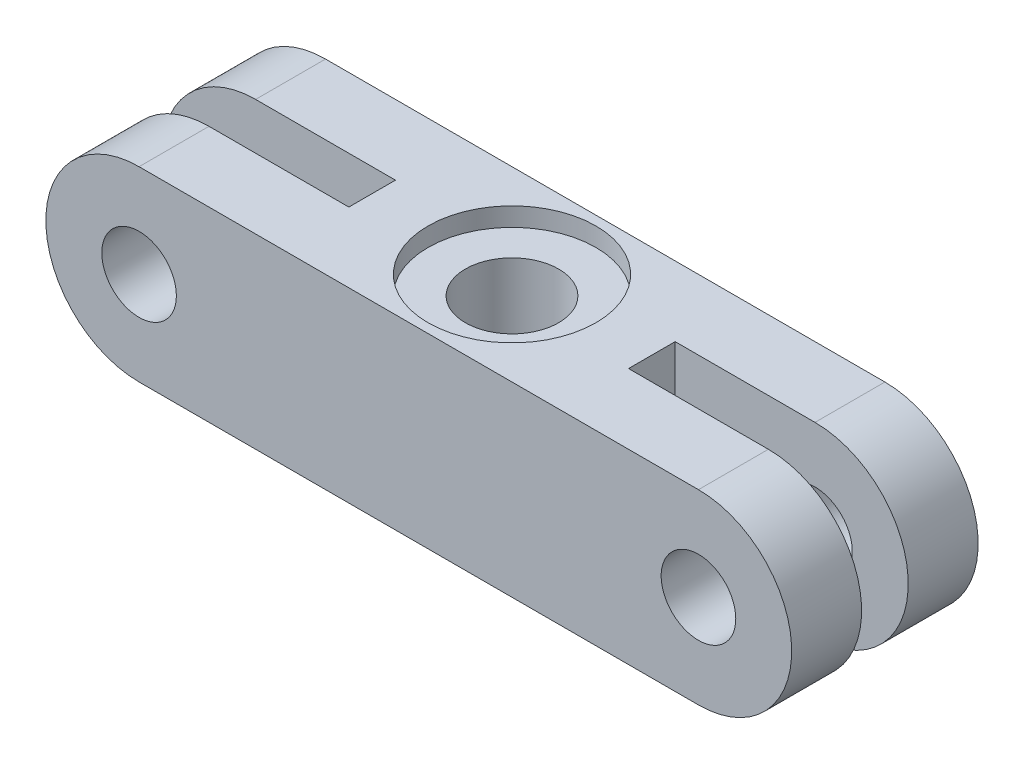
from build123d import *

# Parameters (mm, degrees)
LINK_PROFILE_SKETCH_R           = 4
LINK_BODY_DEPTH                 = 10
END_CLEVIS_SLOTS_5MM_DEPTH      = 46.82575695
END_CLEVIS_SLOTS_5MM_DEPTH_BACK = 46.82575695
END_SLOTS_SKETCH_W              = 25
END_SLOTS_SKETCH_H              = 5
CENTRE_HOLE_10_DEPTH            = 46.82575695
CENTRE_HOLE_10_DEPTH_BACK       = 46.82575695
CENTRE_HOLE_SKETCH_R            = 5
COUNTERBORE_SKETCH_R            = 9
COUNTERBORE_18X2_DEPTH          = 2


with BuildPart() as part:
    # Link Profile Sketch → Link Body (new, symmetric)
    with BuildSketch(Plane.XY):
        with BuildLine():
            Line((-30, 10), (30, 10))
            ThreePointArc((30, 10), (40, 0), (30, -10))
            Line((30, -10), (-30, -10))
            ThreePointArc((-30, -10), (-40, 0), (-30, 10))
        make_face()
        with Locations((-30, 0)):
            Circle(LINK_PROFILE_SKETCH_R, mode=Mode.SUBTRACT)
        with Locations((30, 0)):
            Circle(LINK_PROFILE_SKETCH_R, mode=Mode.SUBTRACT)
    extrude(amount=LINK_BODY_DEPTH, both=True)

    # End Slots Sketch → End Clevis Slots 5mm (cut, two sides: drawn at the far end of the back side and taken through both)
    with BuildSketch(Plane(origin=(0, 10, 0), x_dir=(1, 0, 0), z_dir=(0, 1, 0)).offset(-END_CLEVIS_SLOTS_5MM_DEPTH_BACK)):
        with Locations((-27.5, 0)):
            Rectangle(END_SLOTS_SKETCH_W, END_SLOTS_SKETCH_H)
        with Locations((27.5, 0)):
            Rectangle(END_SLOTS_SKETCH_W, END_SLOTS_SKETCH_H)
    extrude(amount=END_CLEVIS_SLOTS_5MM_DEPTH + END_CLEVIS_SLOTS_5MM_DEPTH_BACK, mode=Mode.SUBTRACT)

    # Centre Hole Sketch → Centre Hole Ø10 (cut, two sides: drawn at the far end of the back side and taken through both)
    with BuildSketch(Plane(origin=(0, 10, 0), x_dir=(1, 0, 0), z_dir=(0, 1, 0)).offset(-CENTRE_HOLE_10_DEPTH_BACK)):
        with Locations(Location((0, 0, 0), (0, 0, 180))):
            Circle(CENTRE_HOLE_SKETCH_R)
    extrude(amount=CENTRE_HOLE_10_DEPTH + CENTRE_HOLE_10_DEPTH_BACK, mode=Mode.SUBTRACT)

    # Counterbore Sketch → Counterbore Ø18x2 (cut)
    with BuildSketch(Plane(origin=(0, 10, 0), x_dir=(1, 0, 0), z_dir=(0, 1, 0))):
        with Locations(Location((0, 0, 0), (0, 0, 180))):
            Circle(COUNTERBORE_SKETCH_R)
    extrude(amount=-COUNTERBORE_18X2_DEPTH, mode=Mode.SUBTRACT)


solid = part.part
